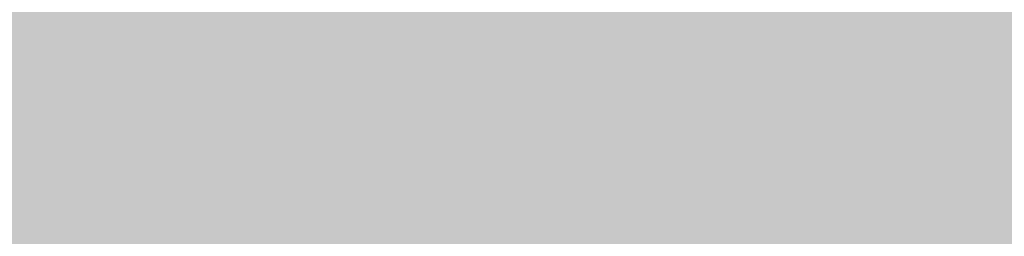
# Model space of a CAD drawing. Units: feet. Extents: x 3168 to 4724, y 827 to 1477.
# Tile 101 of 256: x 3277.376 to 3284.479, y 1096.781 to 1098.344. Entities that reach past the tile are written whole.
import ezdxf

# ---------------------------------------------------------------- set-up
doc = ezdxf.new("R2010")
doc.units = ezdxf.units.FT
doc.layers.add('A-ELEV-PATT', color=8, linetype='Continuous', lineweight=13)

msp = doc.modelspace()

# ---------------------------------------------------------------- hatches: boundary and pattern name
at = {"layer": 'A-ELEV-PATT'}
h = msp.add_hatch(color=256, dxfattribs=at)
h.dxf.hatch_style = 1
edge = h.paths.add_edge_path()
edge.add_ellipse((3552.9058, 979.2201), major_axis=(36.7449, 0), ratio=0.4848485, start_angle=0, end_angle=360)
edge = h.paths.add_edge_path()
edge.add_ellipse((3559.8916, 929.2523), major_axis=(36.7449, 0), ratio=0.4848485, start_angle=0, end_angle=360)
edge = h.paths.add_edge_path()
edge.add_line((3299.3168, 1198.6061), (3479.9167, 1198.6061))
edge.add_line((3479.9167, 1198.6061), (3479.9167, 1209.8686))
edge.add_spline(control_points=[(3479.9167, 1209.8686), (3464.3012, 1209.8686), (3448.6856, 1209.8686), (3410.9491, 1209.8686), (3388.8282, 1209.8686), (3355.6469, 1209.8686), (3344.5864, 1209.8686), (3327.9957, 1209.8686), (3322.4655, 1209.8686), (3314.1702, 1209.8686), (3311.4051, 1209.8686), (3307.2574, 1209.8686), (3305.8748, 1209.8686), (3303.801, 1209.8686), (3303.1097, 1209.8686), (3302.0728, 1209.8686), (3301.7272, 1209.8686), (3301.2087, 1209.8686), (3301.0359, 1209.8686), (3300.7767, 1209.8686), (3300.6903, 1209.8686), (3300.5606, 1209.8686), (3300.5174, 1209.8686), (3300.4526, 1209.8686), (3300.431, 1209.8686), (3300.3986, 1209.8686), (3300.3878, 1209.8686), (3300.3662, 1209.8686), (3300.3457, 1209.8686), (3300.3455, 1209.8686), (3300.3455, 1209.8686), (3300.3433, 1209.8686), (3300.3411, 1209.8686), (3300.3379, 1209.8686), (3300.3368, 1209.8686), (3300.3339, 1209.8686), (3300.3321, 1209.8686), (3300.3255, 1209.8686), (3300.3207, 1209.8686), (3300.3109, 1209.8686), (3300.306, 1209.8686), (3300.2905, 1209.8686), (3300.28, 1209.8686), (3300.2324, 1209.8688), (3300.1953, 1209.869), (3299.9511, 1209.8706), (3299.7448, 1209.8743), (3299.4368, 1209.8833), (3299.3344, 1209.8868), (3299.1811, 1209.8929), (3299.13, 1209.8951), (3298.6522, 1209.9168), (3298.2295, 1209.9457), (3297.6016, 1210.0024), (3297.3934, 1210.0235), (3297.0827, 1210.0583), (3296.9793, 1210.0705), (3296.293, 1210.1549), (3295.7181, 1210.2434), (3294.8687, 1210.3989), (3294.5877, 1210.4545), (3294.1693, 1210.5433), (3294.0304, 1210.5739), (3291.7071, 1211.1012), (3289.6536, 1211.8134), (3285.7763, 1213.564), (3283.9514, 1214.6035), (3280.5122, 1216.9801), (3278.8972, 1218.3176), (3276.3799, 1220.8295), (3275.416, 1221.9177), (3274.0393, 1223.7077), (3273.581, 1224.3495), (3273.1432, 1225.0163)], knot_values=[39.119033, 39.119033, 39.119033, 39.119033, 39.286353, 39.286353, 39.523379, 39.523379, 39.641892, 39.641892, 39.701148, 39.701148, 39.730777, 39.730777, 39.745591, 39.745591, 39.752998, 39.752998, 39.756701, 39.756701, 39.758553, 39.758553, 39.759479, 39.759479, 39.759942, 39.759942, 39.760173, 39.760173, 39.760289, 39.760289, 39.760405, 39.760405, 39.760463, 39.760463, 39.763389, 39.763389, 39.764851, 39.764851, 39.767304, 39.767304, 39.773825, 39.773825, 39.78057, 39.78057, 39.79477, 39.79477, 39.845194, 39.845194, 40.126715, 40.126715, 40.267476, 40.267476, 40.337856, 40.337856, 40.927023, 40.927023, 41.221606, 41.221606, 41.368898, 41.368898, 42.202622, 42.202622, 42.619485, 42.619485, 42.827916, 42.827916, 46.118323, 46.118323, 49.408731, 49.408731, 52.699139, 52.699139, 54.927489, 54.927489, 56.104228, 56.104228, 56.104228, 56.104228], weights=[1, 1, 1, 1, 1, 1, 1, 1, 1, 1, 1, 1, 1, 1, 1, 1, 1, 1, 1, 1, 1, 1, 1, 1, 1, 1, 1, 1, 1, 1, 1, 1, 1, 1, 1, 1, 1, 1, 1, 1, 1, 1, 1, 1, 1, 1, 1, 1, 1, 1, 1, 1, 1, 1, 1, 1, 1, 1, 1, 1, 1, 1, 1, 1, 1, 1, 1, 1, 1, 1, 1, 1, 1, 1], degree=3, periodic=0)
edge.add_line((3273.1432, 1225.0163), (3273.1432, 1099.0163))
edge.add_line((3273.1432, 1099.0163), (3299.3168, 1099.0163))
edge.add_line((3299.3168, 1099.0163), (3299.3168, 1198.6061))
edge = h.paths.add_edge_path()
edge.add_line((3304.7584, 1324.1581), (3479.9167, 1324.1581))
edge.add_line((3479.9167, 1324.1581), (3479.9167, 1335.7146))
edge.add_line((3479.9167, 1335.7146), (3269.1616, 1335.7146))
edge.add_spline(control_points=[(3269.1616, 1335.7146), (3264.0242, 1335.7146), (3258.3641, 1328.9582), (3259.2643, 1323.9003)], knot_values=[0, 0, 0, 0, 15.412191, 15.412191, 15.412191, 15.412191], degree=3, periodic=0)
edge.add_line((3259.2643, 1323.9003), (3265.5168, 1288.7691))
edge.add_line((3265.5168, 1288.7691), (3275.2651, 1261.5456))
edge.add_line((3275.2651, 1261.5456), (3304.7584, 1261.5456))
edge.add_line((3304.7584, 1261.5456), (3304.7584, 1324.1581))
h = msp.add_hatch(color=256, dxfattribs=at)
h.dxf.hatch_style = 1
h.paths.add_polyline_path([(3384.5252, 1099.0163), (3335.0292, 1099.0163), (3299.3168, 1099.0163), (3273.1432, 1099.0163), (3217.5654, 1099.0163), (3168.0693, 827.1163), (3335.0292, 827.1163)])

doc.saveas('drawing.dxf')
